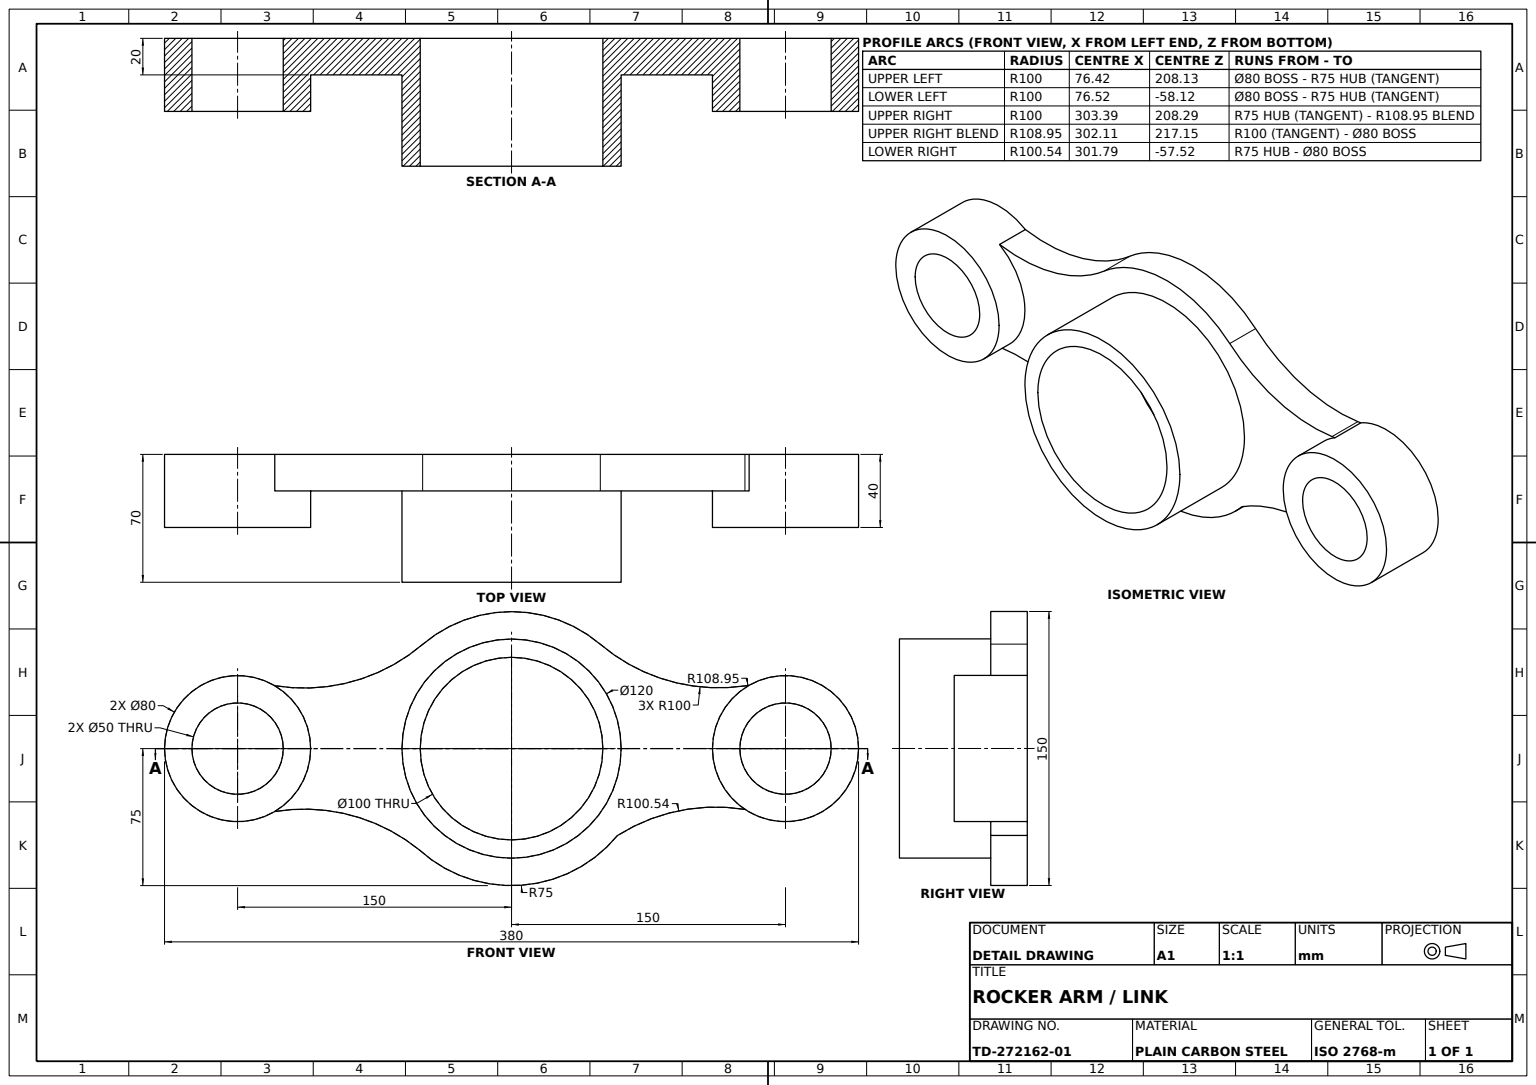
from build123d import *

# Parameters (mm, degrees)
LINK_PLATE_DEPTH      = 20
CENTER_BOSS_SKETCH_R  = 60
CENTER_BOSS_120_DEPTH = 50
CENTER_BORE_SKETCH_R  = 50
CENTER_BORE_100_DEPTH = 70
END_BOSS_A_SKETCH_R   = 40
END_BOSS_A_80_DEPTH   = 20
END_BOSS_B_SKETCH_R   = 40
END_BOSS_B_80_DEPTH   = 20
END_BORES_SKETCH_R    = 25
END_BORES_2X_50_DEPTH = 40


with BuildPart() as part:
    # Link Profile Sketch → Link Plate (new body)
    with BuildSketch(Plane.XY):
        with BuildLine():
            ThreePointArc((-129.642270948, 34.432003541), (-190, 0), (-129.642270948, -34.432003541))
            ThreePointArc((-129.642270948, -34.432003541), (-87.851681721, -36.458860817), (-50.548209333, -55.406484578))
            ThreePointArc((-50.548209333, -55.406484578), (5.374732367, -74.807167116), (57.949801632, -47.611138306))
            ThreePointArc((57.949801632, -47.611138306), (91.552609541, -34.039548838), (127.784288058, -33.263525714))
            ThreePointArc((127.784288058, -33.263525714), (189.977010396, -1.355964531), (130.089258317, 34.692396366))
            ThreePointArc((130.089258317, 34.692396366), (128.937737844, 34.506028192), (127.784288058, 34.331999196))
            ThreePointArc((127.784288058, 34.331999196), (85.734256685, 37.193020101), (48.597851254, 57.124853204))
            ThreePointArc((48.597851254, 57.124853204), (-0.052113987, 74.999981894), (-48.677191075, 57.057261317))
            ThreePointArc((-48.677191075, 57.057261317), (-86.6667217, 36.823333055), (-129.642270948, 34.432003541))
        make_face()
    extrude(amount=LINK_PLATE_DEPTH)

    # Center Boss Sketch → Center Boss Ø120 (add)
    with BuildSketch(Plane.XY.offset(20)):
        Circle(CENTER_BOSS_SKETCH_R)
    extrude(amount=CENTER_BOSS_120_DEPTH)

    # Center Bore Sketch → Center Bore Ø100 (cut)
    with BuildSketch(Plane.XY.offset(70)):
        Circle(CENTER_BORE_SKETCH_R)
    extrude(amount=-CENTER_BORE_100_DEPTH, mode=Mode.SUBTRACT)

    # End Boss A Sketch → End Boss A Ø80 (add)
    with BuildSketch(Plane.XY.offset(20)):
        with Locations(Location((-150, 0, 0), (0, 0, 300.593464185))):
            Circle(END_BOSS_A_SKETCH_R)
    extrude(amount=END_BOSS_A_80_DEPTH)

    # End Boss B Sketch → End Boss B Ø80 (add)
    with BuildSketch(Plane.XY.offset(20)):
        with Locations(Location((150, 0, 0), (0, 0, 236.26222597))):
            Circle(END_BOSS_B_SKETCH_R)
    extrude(amount=END_BOSS_B_80_DEPTH)

    # End Bores Sketch → End Bores 2xØ50 (cut)
    with BuildSketch(Plane.XY.offset(40)):
        with Locations((-150, 0)):
            Circle(END_BORES_SKETCH_R)
        with Locations((150, 0)):
            Circle(END_BORES_SKETCH_R)
    extrude(amount=-END_BORES_2X_50_DEPTH, mode=Mode.SUBTRACT)


solid = part.part
